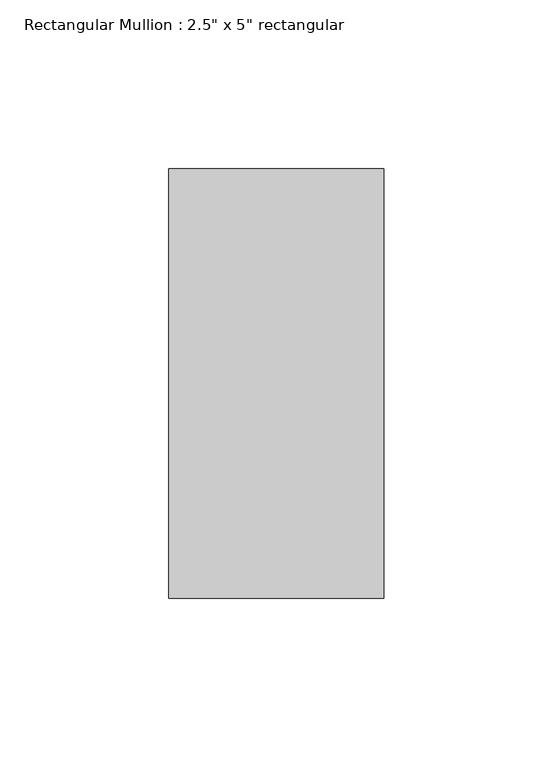
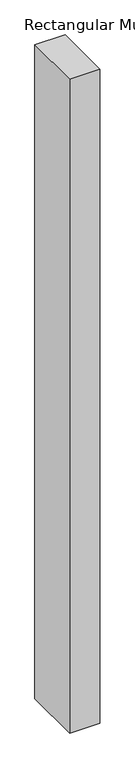
"""IFC4 building model written with IfcOpenShell, lengths in millimetres: member geometry."""

from ifc_helpers import new_model, si_unit, frame, origin, place, context, project, spatial, polyline, outline, extrude, source, transform, mapped, element, save


def member_b57d713a(model_context):
    return source(origin(), model_context, "Body", "SweptSolid", [
        extrude(outline(polyline([(0.0, 63.5), (0.0, -63.5), (-63.5, -63.5), (-63.5, 63.5), (0.0, 63.5)])), frame((0.0, 0.0, -1457.1797686), z_axis=(0.0, 0.0, 1.0), x_axis=(1.0, 0.0, 0.0)), (0.0, 0.0, 1.0), 1457.1797686),
    ])


if __name__ == "__main__":
    model = new_model("IFC4")
    model_context = context("Model", 3, world=origin())
    ifc_project = project(units=[si_unit("LENGTHUNIT", "METRE", prefix="MILLI")], contexts=[model_context])
    site = spatial("IfcSite", under=ifc_project)
    building = spatial("IfcBuilding", under=site)
    placement = place(None, origin())
    member_shape = member_b57d713a(model_context)
    element("IfcMember", 1, ObjectType="Rectangular Mullion : 2.5\" x 5\" rectangular", at=placement, inside=building, context=model_context, shape_type="MappedRepresentation", body=[
        mapped(member_shape, transform((0.0, 0.0, 0.0), x_axis=(1.0, 0.0, 0.0), y_axis=(0.0, 1.0, 0.0), z_axis=(0.0, 0.0, 1.0))),
    ])
    save(model, "model.ifc")

# Revit data of these elements
# Type "Rectangular Mullion : 2.5\" x 5\" rectangular"
#   built-in parameter 1007304 = 0.416667 (stored number, unit not read)
#   built-in parameter 1007301 = 0.104167 (stored number, unit not read)
#   built-in parameter 1007300 = 0.104167 (stored number, unit not read)
# Element 1 (IfcMember, "Rectangular Mullion : 2.5\" x 5\" rectangular")
#   Materials on its faces: "Aluminum"
# Materials
#   "Aluminum": class "Metal", colour RGB 247 247 247, transparency 0, Description = "Aluminum 6061", Cost = 0
